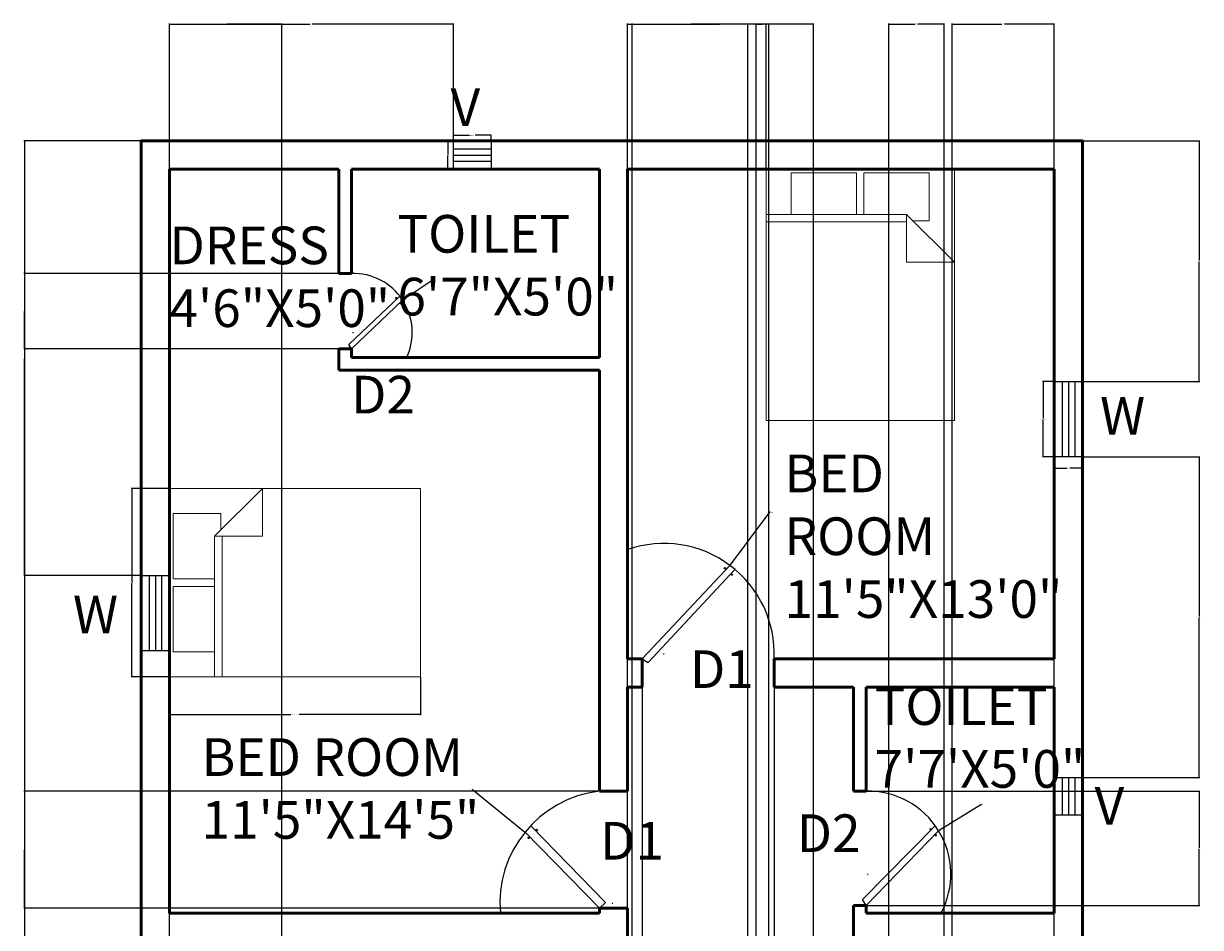
# Model space of a CAD drawing. Units: inches. Extents: x -15 to 361, y -684 to 58.
# Tile 3 of 3: x -15 to 361, y -230 to 58. Entities that reach past the tile are written whole.
import ezdxf

# ---------------------------------------------------------------- set-up
doc = ezdxf.new("R2010")
doc.units = ezdxf.units.IN
doc.header["$MEASUREMENT"] = 0
for name, color, linetype, lineweight in [('A-ANNO-DIMS', 2, 'Continuous', 18), ('A-ANNO-TEXT', 7, 'Continuous', 18), ('A-AREA-IDEN', 7, 'Continuous', 25), ('A-DOOR', 3, 'Continuous', 25), ('A-FURN', 8, 'Continuous', 18), ('A-GLAZ', 4, 'Continuous', 25), ('A-WALL', 7, 'Continuous', 50)]:
    doc.layers.add(name, color=color, linetype=linetype, lineweight=lineweight)
doc.styles.get("Standard").update_dxf_attribs({"font": 'arial.ttf'})
doc.dimstyles.get("Standard").update_dxf_attribs({"dimtxt": 0.18, "dimasz": 0.18, "dimexe": 0.18, "dimexo": 0.0625, "dimgap": 0.09, "dimtad": 0, "dimtih": 1, "dimtoh": 1, "dimdec": 4, "dimzin": 0, "dimdsep": 46, "dimtxsty": 'Standard', "dimcen": 0.09, "dimadec": 0, "dimazin": 0, "dimtfac": 1, "dimtdec": 4, "dimtofl": 0, "dimtmove": 0, "dimatfit": 3, "dimfxl": 1, "dimtolj": 1, "dimtzin": 0, "dimarcsym": 0})

# ---------------------------------------------------------------- blocks, each defined once
blk = doc.blocks.new('Bed - Queen')
for p, q in [((0, -80.00003), (0, 0)), ((0, 0), (59.99999, 0)), ((59.99999, 0), (59.99999, -80.00003)), ((7.99999, -1.2), (28.79998, -1.2)), ((7.99999, -14.4), (7.99999, -1.2)), ((28.79998, -1.2), (28.79998, -14.4)), ((31.19999, -1.2), (51.99999, -1.2)), ((31.19999, -14.4), (31.19999, -1.2)), ((51.99999, -1.2), (51.99999, -16.4)), ((0, -14.4), (44.8, -14.4)), ((59.99999, -29.6), (44.8, -14.4)), ((44.8, -14.4), (44.8, -29.6)), ((44.8, -16.8), (0, -16.8)), ((51.99999, -16.4), (46.79936, -16.4)), ((44.8, -29.6), (59.99999, -29.6)), ((59.99999, -80.00003), (0, -80.00003))]:
    blk.add_line(p, q)
blk = doc.blocks.new('WIN-24IN')
for p, q in [((0, 6.5), (24, 6.5)), ((0, 4.5), (24, 4.5)), ((0, 2.5), (24, 2.5))]:
    blk.add_line(p, q)
blk.add_lwpolyline([(0, 9), (24, 9), (24, 0), (0, 0)], close=True)
blk = doc.blocks.new('VENT-12IN')
for p, q in [((0, 6.5), (12, 6.5)), ((0, 4.5), (12, 4.5)), ((0, 2.5), (12, 2.5))]:
    blk.add_line(p, q)
blk.add_lwpolyline([(0, 9), (12, 9), (12, 0), (0, 0)], close=True)
blk = doc.blocks.new('*D9')
at = {"layer": 'A-ANNO-DIMS', "color": 0, "lineweight": -2, "transparency": 16777216}
for p, q in [((313.87, -56.3), (310.15, -56.3)), ((310.33, -56.48), (310.33, -68.12)), ((310.33, -80.12), (310.33, -68.48)), ((313.87, -80.3), (310.15, -80.3))]:
    blk.add_line(p, q, dxfattribs=at)
at = {"layer": 'A-ANNO-DIMS', "color": 0, "transparency": 16777216}
for points in [[(310.3, -56.48), (310.36, -56.48), (310.33, -56.3)], [(310.3, -80.12), (310.36, -80.12), (310.33, -80.3)]]:
    blk.add_solid(points, dxfattribs=at)
at = {"layer": 'Defpoints', "color": 0, "transparency": 16777216}
for p in [(313.93, -56.3), (310.33, -80.3), (313.93, -80.3)]:
    blk.add_point(p, dxfattribs=at)
at = {"layer": 'A-ANNO-DIMS', "color": 0, "transparency": 16777216, "insert": (310.33, -68.3), "char_height": 0.18, "attachment_point": 5}
blk.add_mtext('\\A1;WINDOW 24 TYP.', dxfattribs=at)
blk = doc.blocks.new('*D10')
at = {"layer": 'A-ANNO-DIMS', "color": 0, "lineweight": -2, "transparency": 16777216}
for p, q in [((313.93, -80.36), (313.93, -84.08)), ((322.93, -80.36), (322.93, -84.08)), ((314.11, -83.9), (317.97, -83.9)), ((322.75, -83.9), (318.89, -83.9))]:
    blk.add_line(p, q, dxfattribs=at)
at = {"layer": 'A-ANNO-DIMS', "color": 0, "transparency": 16777216}
for points in [[(314.11, -83.87), (314.11, -83.93), (313.93, -83.9)], [(322.75, -83.87), (322.75, -83.93), (322.93, -83.9)]]:
    blk.add_solid(points, dxfattribs=at)
at = {"layer": 'Defpoints', "color": 0, "transparency": 16777216}
for p in [(313.93, -80.3), (322.93, -80.3), (322.93, -83.9)]:
    blk.add_point(p, dxfattribs=at)
at = {"layer": 'A-ANNO-DIMS', "color": 0, "transparency": 16777216, "insert": (318.43, -83.9), "char_height": 0.18, "attachment_point": 5}
blk.add_mtext('\\A1;9 TYP.', dxfattribs=at)
blk = doc.blocks.new('*D11')
at = {"layer": 'A-ANNO-DIMS', "color": 0, "lineweight": -2, "transparency": 16777216}
for p, q in [((122.4, 20.37), (122.4, 22.29)), ((122.58, 22.11), (127.5, 22.11)), ((134.22, 22.11), (129.31, 22.11)), ((134.4, 20.37), (134.4, 22.29))]:
    blk.add_line(p, q, dxfattribs=at)
at = {"layer": 'A-ANNO-DIMS', "color": 0, "transparency": 16777216}
for points in [[(122.58, 22.14), (122.58, 22.08), (122.4, 22.11)], [(134.22, 22.14), (134.22, 22.08), (134.4, 22.11)]]:
    blk.add_solid(points, dxfattribs=at)
at = {"layer": 'Defpoints', "color": 0, "transparency": 16777216}
for p in [(122.4, 20.31), (134.4, 22.11), (134.4, 20.31)]:
    blk.add_point(p, dxfattribs=at)
at = {"layer": 'A-ANNO-DIMS', "color": 0, "transparency": 16777216, "insert": (128.4, 22.11), "char_height": 0.18, "attachment_point": 5}
blk.add_mtext('\\A1;VENT 12 TYP.', dxfattribs=at)
blk = doc.blocks.new('*D12')
at = {"layer": 'A-ANNO-DIMS', "color": 0, "lineweight": -2, "transparency": 16777216}
for p, q in [((122.34, 20.31), (120.42, 20.31)), ((120.6, 20.13), (120.6, 15.99)), ((120.6, 11.49), (120.6, 15.63)), ((122.34, 11.31), (120.42, 11.31))]:
    blk.add_line(p, q, dxfattribs=at)
at = {"layer": 'A-ANNO-DIMS', "color": 0, "transparency": 16777216}
for points in [[(120.57, 20.13), (120.63, 20.13), (120.6, 20.31)], [(120.57, 11.49), (120.63, 11.49), (120.6, 11.31)]]:
    blk.add_solid(points, dxfattribs=at)
at = {"layer": 'Defpoints', "color": 0, "transparency": 16777216}
for p in [(120.6, 20.31), (122.4, 20.31), (122.4, 11.31)]:
    blk.add_point(p, dxfattribs=at)
at = {"layer": 'A-ANNO-DIMS', "color": 0, "transparency": 16777216, "insert": (120.6, 15.81), "char_height": 0.18, "attachment_point": 5}
blk.add_mtext('\\A1;9 TYP.', dxfattribs=at)
blk = doc.blocks.new('*D13')
at = {"layer": 'A-ANNO-DIMS', "color": 0, "lineweight": -2, "transparency": 16777216}
for p, q in [((31.93, -150.43), (31.93, -162.55)), ((111.93, -150.43), (111.93, -162.55)), ((32.11, -162.37), (70.62, -162.37)), ((111.75, -162.37), (73.23, -162.37))]:
    blk.add_line(p, q, dxfattribs=at)
at = {"layer": 'A-ANNO-DIMS', "color": 0, "transparency": 16777216}
for points in [[(32.11, -162.34), (32.11, -162.4), (31.93, -162.37)], [(111.75, -162.34), (111.75, -162.4), (111.93, -162.37)]]:
    blk.add_solid(points, dxfattribs=at)
at = {"layer": 'Defpoints', "color": 0, "transparency": 16777216}
for p in [(31.93, -150.37), (111.93, -150.37), (31.93, -162.37)]:
    blk.add_point(p, dxfattribs=at)
at = {"layer": 'A-ANNO-DIMS', "color": 0, "transparency": 16777216, "insert": (71.93, -162.37), "char_height": 0.18, "attachment_point": 5}
blk.add_mtext('\\A1;QUEEN BED 80 TYP.', dxfattribs=at)
blk = doc.blocks.new('*D14')
at = {"layer": 'A-ANNO-DIMS', "color": 0, "lineweight": -2, "transparency": 16777216}
for p, q in [((31.87, -90.37), (19.75, -90.37)), ((19.93, -90.55), (19.93, -120.18)), ((19.93, -150.19), (19.93, -120.55)), ((31.87, -150.37), (19.75, -150.37))]:
    blk.add_line(p, q, dxfattribs=at)
at = {"layer": 'A-ANNO-DIMS', "color": 0, "transparency": 16777216}
for points in [[(19.9, -90.55), (19.96, -90.55), (19.93, -90.37)], [(19.9, -150.19), (19.96, -150.19), (19.93, -150.37)]]:
    blk.add_solid(points, dxfattribs=at)
at = {"layer": 'Defpoints', "color": 0, "transparency": 16777216}
for p in [(19.93, -90.37), (31.93, -90.37), (31.93, -150.37)]:
    blk.add_point(p, dxfattribs=at)
at = {"layer": 'A-ANNO-DIMS', "color": 0, "transparency": 16777216, "insert": (19.93, -120.37), "char_height": 0.18, "attachment_point": 5}
blk.add_mtext('\\A1;60 TYP.', dxfattribs=at)
blk = doc.blocks.new('*D24')
at = {"layer": 'A-ANNO-DIMS', "color": 0, "lineweight": -2, "transparency": 16777216}
for p, q in [((22.87, 20.31), (-14.45, 20.31)), ((-14.27, 20.13), (-14.27, -309.51)), ((-14.27, -639.51), (-14.27, -309.87)), ((22.87, -639.69), (-14.45, -639.69))]:
    blk.add_line(p, q, dxfattribs=at)
at = {"layer": 'A-ANNO-DIMS', "color": 0, "transparency": 16777216}
for points in [[(-14.3, 20.13), (-14.24, 20.13), (-14.27, 20.31)], [(-14.3, -639.51), (-14.24, -639.51), (-14.27, -639.69)]]:
    blk.add_solid(points, dxfattribs=at)
at = {"layer": 'Defpoints', "color": 0, "transparency": 16777216}
for p in [(-14.27, 20.31), (22.93, 20.31), (22.93, -639.69)]:
    blk.add_point(p, dxfattribs=at)
at = {"layer": 'A-ANNO-DIMS', "color": 0, "transparency": 16777216, "insert": (-14.27, -309.69), "char_height": 0.18, "attachment_point": 5}
blk.add_mtext('\\A1;660', dxfattribs=at)
blk = doc.blocks.new('*D25')
at = {"layer": 'A-ANNO-DIMS', "color": 0, "lineweight": -2, "transparency": 16777216}
for p, q in [((31.93, 11.37), (31.93, 57.69)), ((32.11, 57.51), (76.77, 57.51)), ((122.22, 57.51), (77.56, 57.51)), ((122.4, 11.37), (122.4, 57.69))]:
    blk.add_line(p, q, dxfattribs=at)
at = {"layer": 'A-ANNO-DIMS', "color": 0, "transparency": 16777216}
for points in [[(32.11, 57.54), (32.11, 57.48), (31.93, 57.51)], [(122.22, 57.54), (122.22, 57.48), (122.4, 57.51)]]:
    blk.add_solid(points, dxfattribs=at)
at = {"layer": 'Defpoints', "color": 0, "transparency": 16777216}
for p in [(122.4, 57.51), (31.93, 11.31), (122.4, 11.31)]:
    blk.add_point(p, dxfattribs=at)
at = {"layer": 'A-ANNO-DIMS', "color": 0, "transparency": 16777216, "insert": (77.16, 57.51), "char_height": 0.18, "attachment_point": 5}
blk.add_mtext('\\A1;90.47', dxfattribs=at)
blk = doc.blocks.new('*D26')
at = {"layer": 'A-ANNO-DIMS', "color": 0, "lineweight": -2, "transparency": 16777216}
for p, q in [((322.99, 20.31), (360.31, 20.31)), ((360.13, 20.13), (360.13, -17.81)), ((360.13, -56.12), (360.13, -18.18)), ((322.99, -56.3), (360.31, -56.3))]:
    blk.add_line(p, q, dxfattribs=at)
at = {"layer": 'A-ANNO-DIMS', "color": 0, "transparency": 16777216}
for points in [[(360.1, 20.13), (360.16, 20.13), (360.13, 20.31)], [(360.1, -56.12), (360.16, -56.12), (360.13, -56.3)]]:
    blk.add_solid(points, dxfattribs=at)
at = {"layer": 'Defpoints', "color": 0, "transparency": 16777216}
for p in [(322.93, 20.31), (322.93, -56.3), (360.13, -56.3)]:
    blk.add_point(p, dxfattribs=at)
at = {"layer": 'A-ANNO-DIMS', "color": 0, "transparency": 16777216, "insert": (360.13, -18), "char_height": 0.18, "attachment_point": 5}
blk.add_mtext('\\A1;76.61', dxfattribs=at)
blk = doc.blocks.new('*D27')
at = {"layer": 'A-ANNO-DIMS', "color": 0, "lineweight": -2, "transparency": 16777216}
for p, q in [((322.99, -80.3), (360.31, -80.3)), ((360.13, -80.48), (360.13, -131.21)), ((360.13, -182.3), (360.13, -131.57)), ((322.99, -182.48), (360.31, -182.48))]:
    blk.add_line(p, q, dxfattribs=at)
at = {"layer": 'A-ANNO-DIMS', "color": 0, "transparency": 16777216}
for points in [[(360.1, -80.48), (360.16, -80.48), (360.13, -80.3)], [(360.1, -182.3), (360.16, -182.3), (360.13, -182.48)]]:
    blk.add_solid(points, dxfattribs=at)
at = {"layer": 'Defpoints', "color": 0, "transparency": 16777216}
for p in [(322.93, -80.3), (322.93, -182.48), (360.13, -182.48)]:
    blk.add_point(p, dxfattribs=at)
at = {"layer": 'A-ANNO-DIMS', "color": 0, "transparency": 16777216, "insert": (360.13, -131.39), "char_height": 0.18, "attachment_point": 5}
blk.add_mtext('\\A1;102.18', dxfattribs=at)
blk = doc.blocks.new('*D31')
at = {"layer": 'A-ANNO-DIMS', "color": 0, "lineweight": -2, "transparency": 16777216}
for p, q in [((177.93, -549.63), (177.93, 57.69)), ((178.11, 57.51), (207.18, 57.51)), ((237.04, 57.51), (207.97, 57.51)), ((237.22, -549.63), (237.22, 57.69))]:
    blk.add_line(p, q, dxfattribs=at)
at = {"layer": 'A-ANNO-DIMS', "color": 0, "transparency": 16777216}
for points in [[(178.11, 57.54), (178.11, 57.48), (177.93, 57.51)], [(237.04, 57.54), (237.04, 57.48), (237.22, 57.51)]]:
    blk.add_solid(points, dxfattribs=at)
at = {"layer": 'Defpoints', "color": 0, "transparency": 16777216}
for p in [(237.22, 57.51), (177.93, -549.69), (237.22, -549.69)]:
    blk.add_point(p, dxfattribs=at)
at = {"layer": 'A-ANNO-DIMS', "color": 0, "transparency": 16777216, "insert": (207.57, 57.51), "char_height": 0.18, "attachment_point": 5}
blk.add_mtext('\\A1;59.29', dxfattribs=at)
blk = doc.blocks.new('*D32')
at = {"layer": 'A-ANNO-DIMS', "color": 0, "lineweight": -2, "transparency": 16777216}
for p, q in [((31.93, -396.63), (31.93, 57.69)), ((32.11, 57.51), (49.42, 57.51)), ((67.52, 57.51), (50.21, 57.51)), ((67.7, -396.63), (67.7, 57.69))]:
    blk.add_line(p, q, dxfattribs=at)
at = {"layer": 'A-ANNO-DIMS', "color": 0, "transparency": 16777216}
for points in [[(32.11, 57.54), (32.11, 57.48), (31.93, 57.51)], [(67.52, 57.54), (67.52, 57.48), (67.7, 57.51)]]:
    blk.add_solid(points, dxfattribs=at)
at = {"layer": 'Defpoints', "color": 0, "transparency": 16777216}
for p in [(67.7, 57.51), (31.93, -396.69), (67.7, -396.69)]:
    blk.add_point(p, dxfattribs=at)
at = {"layer": 'A-ANNO-DIMS', "color": 0, "transparency": 16777216, "insert": (49.81, 57.51), "char_height": 0.18, "attachment_point": 5}
blk.add_mtext('\\A1;35.77', dxfattribs=at)
blk = doc.blocks.new('*D33')
at = {"layer": 'A-ANNO-DIMS', "color": 0, "lineweight": -2, "transparency": 16777216}
for p, q in [((22.87, 20.31), (-14.45, 20.31)), ((-14.27, 20.13), (-14.27, -48.7)), ((-14.27, -117.9), (-14.27, -49.07)), ((22.87, -118.08), (-14.45, -118.08))]:
    blk.add_line(p, q, dxfattribs=at)
at = {"layer": 'A-ANNO-DIMS', "color": 0, "transparency": 16777216}
for points in [[(-14.3, 20.13), (-14.24, 20.13), (-14.27, 20.31)], [(-14.3, -117.9), (-14.24, -117.9), (-14.27, -118.08)]]:
    blk.add_solid(points, dxfattribs=at)
at = {"layer": 'Defpoints', "color": 0, "transparency": 16777216}
for p in [(22.93, 20.31), (-14.27, -118.08), (22.93, -118.08)]:
    blk.add_point(p, dxfattribs=at)
at = {"layer": 'A-ANNO-DIMS', "color": 0, "transparency": 16777216, "insert": (-14.27, -48.89), "char_height": 0.18, "attachment_point": 5}
blk.add_mtext('\\A1;138.4', dxfattribs=at)
blk = doc.blocks.new('*D36')
at = {"layer": 'A-ANNO-DIMS', "color": 0, "lineweight": -2, "transparency": 16777216}
for p, q in [((85.87, -21.88), (-14.45, -21.88)), ((-14.27, -22.06), (-14.27, -33.7)), ((-14.27, -45.7), (-14.27, -34.06)), ((85.87, -45.88), (-14.45, -45.88))]:
    blk.add_line(p, q, dxfattribs=at)
at = {"layer": 'A-ANNO-DIMS', "color": 0, "transparency": 16777216}
for points in [[(-14.3, -22.06), (-14.24, -22.06), (-14.27, -21.88)], [(-14.3, -45.7), (-14.24, -45.7), (-14.27, -45.88)]]:
    blk.add_solid(points, dxfattribs=at)
at = {"layer": 'Defpoints', "color": 0, "transparency": 16777216}
for p in [(85.93, -21.88), (-14.27, -45.88), (85.93, -45.88)]:
    blk.add_point(p, dxfattribs=at)
at = {"layer": 'A-ANNO-DIMS', "color": 0, "transparency": 16777216, "insert": (-14.27, -33.88), "char_height": 0.18, "attachment_point": 5}
blk.add_mtext('\\A1;24', dxfattribs=at)
blk = doc.blocks.new('*D37')
at = {"layer": 'A-ANNO-DIMS', "color": 0, "lineweight": -2, "transparency": 16777216}
for p, q in [((182.53, -153.75), (182.53, -677.07)), ((224.64, -153.75), (224.64, -677.07)), ((182.71, -676.89), (203.21, -676.89)), ((224.46, -676.89), (203.97, -676.89))]:
    blk.add_line(p, q, dxfattribs=at)
at = {"layer": 'A-ANNO-DIMS', "color": 0, "transparency": 16777216}
for points in [[(182.71, -676.86), (182.71, -676.92), (182.53, -676.89)], [(224.46, -676.86), (224.46, -676.92), (224.64, -676.89)]]:
    blk.add_solid(points, dxfattribs=at)
at = {"layer": 'Defpoints', "color": 0, "transparency": 16777216}
for p in [(182.53, -153.69), (224.64, -153.69), (224.64, -676.89)]:
    blk.add_point(p, dxfattribs=at)
at = {"layer": 'A-ANNO-DIMS', "color": 0, "transparency": 16777216, "insert": (203.59, -676.89), "char_height": 0.18, "attachment_point": 5}
blk.add_mtext('\\A1;42.11', dxfattribs=at)
blk = doc.blocks.new('*D38')
at = {"layer": 'A-ANNO-DIMS', "color": 0, "lineweight": -2, "transparency": 16777216}
for p, q in [((168.87, -186.78), (-14.45, -186.78)), ((-14.27, -186.96), (-14.27, -205.25)), ((-14.27, -223.91), (-14.27, -205.62)), ((168.87, -224.09), (-14.45, -224.09))]:
    blk.add_line(p, q, dxfattribs=at)
at = {"layer": 'A-ANNO-DIMS', "color": 0, "transparency": 16777216}
for points in [[(-14.3, -186.96), (-14.24, -186.96), (-14.27, -186.78)], [(-14.3, -223.91), (-14.24, -223.91), (-14.27, -224.09)]]:
    blk.add_solid(points, dxfattribs=at)
at = {"layer": 'Defpoints', "color": 0, "transparency": 16777216}
for p in [(168.93, -186.78), (-14.27, -224.09), (168.93, -224.09)]:
    blk.add_point(p, dxfattribs=at)
at = {"layer": 'A-ANNO-DIMS', "color": 0, "transparency": 16777216, "insert": (-14.27, -205.44), "char_height": 0.18, "attachment_point": 5}
blk.add_mtext('\\A1;37.31', dxfattribs=at)
blk = doc.blocks.new('*D39')
at = {"layer": 'A-ANNO-DIMS', "color": 0, "lineweight": -2, "transparency": 16777216}
for p, q in [((253.99, -186.78), (360.31, -186.78)), ((360.13, -186.96), (360.13, -204.81)), ((360.13, -223.02), (360.13, -205.17)), ((253.99, -223.2), (360.31, -223.2))]:
    blk.add_line(p, q, dxfattribs=at)
at = {"layer": 'A-ANNO-DIMS', "color": 0, "transparency": 16777216}
for points in [[(360.1, -186.96), (360.16, -186.96), (360.13, -186.78)], [(360.1, -223.02), (360.16, -223.02), (360.13, -223.2)]]:
    blk.add_solid(points, dxfattribs=at)
at = {"layer": 'Defpoints', "color": 0, "transparency": 16777216}
for p in [(253.93, -186.78), (253.93, -223.2), (360.13, -223.2)]:
    blk.add_point(p, dxfattribs=at)
at = {"layer": 'A-ANNO-DIMS', "color": 0, "transparency": 16777216, "insert": (360.13, -204.99), "char_height": 0.18, "attachment_point": 5}
blk.add_mtext('\\A1;36.42', dxfattribs=at)
blk = doc.blocks.new('*D42')
at = {"layer": 'A-ANNO-DIMS', "color": 0, "lineweight": -2, "transparency": 16777216}
for p, q in [((179.42, -396.63), (179.42, 57.69)), ((179.6, 57.51), (197.42, 57.51)), ((216.02, 57.51), (198.21, 57.51)), ((216.2, -396.63), (216.2, 57.69))]:
    blk.add_line(p, q, dxfattribs=at)
at = {"layer": 'A-ANNO-DIMS', "color": 0, "transparency": 16777216}
for points in [[(179.6, 57.54), (179.6, 57.48), (179.42, 57.51)], [(216.02, 57.54), (216.02, 57.48), (216.2, 57.51)]]:
    blk.add_solid(points, dxfattribs=at)
at = {"layer": 'Defpoints', "color": 0, "transparency": 16777216}
for p in [(216.2, 57.51), (179.42, -396.69), (216.2, -396.69)]:
    blk.add_point(p, dxfattribs=at)
at = {"layer": 'A-ANNO-DIMS', "color": 0, "transparency": 16777216, "insert": (197.81, 57.51), "char_height": 0.18, "attachment_point": 5}
blk.add_mtext('\\A1;36.78', dxfattribs=at)
blk = doc.blocks.new('*D44')
at = {"layer": 'A-ANNO-DIMS', "color": 0, "lineweight": -2, "transparency": 16777216}
for p, q in [((281.35, -558.63), (281.35, 57.69)), ((281.53, 57.51), (297.18, 57.51)), ((313.75, 57.51), (298.1, 57.51)), ((313.93, -558.63), (313.93, 57.69))]:
    blk.add_line(p, q, dxfattribs=at)
at = {"layer": 'A-ANNO-DIMS', "color": 0, "transparency": 16777216}
for points in [[(281.53, 57.54), (281.53, 57.48), (281.35, 57.51)], [(313.75, 57.54), (313.75, 57.48), (313.93, 57.51)]]:
    blk.add_solid(points, dxfattribs=at)
at = {"layer": 'Defpoints', "color": 0, "transparency": 16777216}
for p in [(313.93, 57.51), (281.35, -558.69), (313.93, -558.69)]:
    blk.add_point(p, dxfattribs=at)
at = {"layer": 'A-ANNO-DIMS', "color": 0, "transparency": 16777216, "insert": (297.64, 57.51), "char_height": 0.18, "attachment_point": 5}
blk.add_mtext('\\A1;32.575', dxfattribs=at)
blk = doc.blocks.new('*D49')
at = {"layer": 'A-ANNO-DIMS', "color": 0, "lineweight": -2, "transparency": 16777216}
for p, q in [((218.93, -315.63), (218.93, 57.69)), ((219.11, 57.51), (220.78, 57.51)), ((222.75, 57.51), (221.08, 57.51)), ((222.93, -315.63), (222.93, 57.69))]:
    blk.add_line(p, q, dxfattribs=at)
at = {"layer": 'A-ANNO-DIMS', "color": 0, "transparency": 16777216}
for points in [[(219.11, 57.54), (219.11, 57.48), (218.93, 57.51)], [(222.75, 57.54), (222.75, 57.48), (222.93, 57.51)]]:
    blk.add_solid(points, dxfattribs=at)
at = {"layer": 'Defpoints', "color": 0, "transparency": 16777216}
for p in [(222.93, 57.51), (218.93, -315.69), (222.93, -315.69)]:
    blk.add_point(p, dxfattribs=at)
at = {"layer": 'A-ANNO-DIMS', "color": 0, "transparency": 16777216, "insert": (220.93, 57.51), "char_height": 0.18, "attachment_point": 5}
blk.add_mtext('\\A1;4', dxfattribs=at)
blk = doc.blocks.new('*D51')
at = {"layer": 'A-ANNO-DIMS', "color": 0, "lineweight": -2, "transparency": 16777216}
for p, q in [((177.93, 11.37), (177.93, 57.69)), ((178.11, 57.51), (199.53, 57.51)), ((221.88, 57.51), (200.46, 57.51)), ((222.06, 11.37), (222.06, 57.69))]:
    blk.add_line(p, q, dxfattribs=at)
at = {"layer": 'A-ANNO-DIMS', "color": 0, "transparency": 16777216}
for points in [[(178.11, 57.54), (178.11, 57.48), (177.93, 57.51)], [(221.88, 57.54), (221.88, 57.48), (222.06, 57.51)]]:
    blk.add_solid(points, dxfattribs=at)
at = {"layer": 'Defpoints', "color": 0, "transparency": 16777216}
for p in [(177.93, 57.51), (177.93, 11.31), (222.06, 11.31)]:
    blk.add_point(p, dxfattribs=at)
at = {"layer": 'A-ANNO-DIMS', "color": 0, "transparency": 16777216, "insert": (200, 57.51), "char_height": 0.18, "attachment_point": 5}
blk.add_mtext('\\A1;44.135', dxfattribs=at)
blk = doc.blocks.new('*D52')
at = {"layer": 'A-ANNO-DIMS', "color": 0, "lineweight": -2, "transparency": 16777216}
for p, q in [((261.22, -549.63), (261.22, 57.69)), ((261.4, 57.51), (269.54, 57.51)), ((278.6, 57.51), (270.45, 57.51)), ((278.78, -549.63), (278.78, 57.69))]:
    blk.add_line(p, q, dxfattribs=at)
at = {"layer": 'A-ANNO-DIMS', "color": 0, "transparency": 16777216}
for points in [[(261.4, 57.54), (261.4, 57.48), (261.22, 57.51)], [(278.6, 57.54), (278.6, 57.48), (278.78, 57.51)]]:
    blk.add_solid(points, dxfattribs=at)
at = {"layer": 'Defpoints', "color": 0, "transparency": 16777216}
for p in [(278.78, 57.51), (261.22, -549.69), (278.78, -549.69)]:
    blk.add_point(p, dxfattribs=at)
at = {"layer": 'A-ANNO-DIMS', "color": 0, "transparency": 16777216, "insert": (270, 57.51), "char_height": 0.18, "attachment_point": 5}
blk.add_mtext('\\A1;17.564', dxfattribs=at)
blk = doc.blocks.new('*D53')
at = {"layer": 'A-ANNO-DIMS', "color": 0, "lineweight": -2, "transparency": 16777216}
for p, q in [((115.66, -24.17), (106.36, -30.28)), ((115.84, -24.17), (115.66, -24.17)), ((90.37, -40.72), (90.55, -40.72)), ((90.46, -40.81), (90.46, -40.63))]:
    blk.add_line(p, q, dxfattribs=at)
at = {"layer": 'A-ANNO-DIMS', "color": 0, "transparency": 16777216}
blk.add_solid([(106.35, -30.25), (106.38, -30.3), (106.21, -30.38)], dxfattribs=at)
at = {"layer": 'Defpoints', "color": 0, "transparency": 16777216}
for p in [(106.21, -30.38), (90.46, -40.72)]:
    blk.add_point(p, dxfattribs=at)
at = {"layer": 'A-ANNO-DIMS', "color": 0, "transparency": 16777216, "insert": (116.32, -24.17), "char_height": 0.18, "attachment_point": 5}
blk.add_mtext('\\A1;R18.85', dxfattribs=at)
blk = doc.blocks.new('*D54')
at = {"layer": 'A-ANNO-DIMS', "color": 0, "lineweight": -2, "transparency": 16777216}
for p, q in [((223.15, -97.95), (210.64, -114.73)), ((223.33, -97.95), (223.15, -97.95)), ((189.41, -143.07), (189.59, -143.07)), ((189.5, -143.16), (189.5, -142.98))]:
    blk.add_line(p, q, dxfattribs=at)
at = {"layer": 'A-ANNO-DIMS', "color": 0, "transparency": 16777216}
blk.add_solid([(210.62, -114.71), (210.66, -114.75), (210.53, -114.87)], dxfattribs=at)
at = {"layer": 'Defpoints', "color": 0, "transparency": 16777216}
for p in [(210.53, -114.87), (189.5, -143.07)]:
    blk.add_point(p, dxfattribs=at)
at = {"layer": 'A-ANNO-DIMS', "color": 0, "transparency": 16777216, "insert": (223.88, -97.95), "char_height": 0.18, "attachment_point": 5}
blk.add_mtext('\\A1;R35.174', dxfattribs=at)
blk = doc.blocks.new('*D55')
at = {"layer": 'A-ANNO-DIMS', "color": 0, "lineweight": -2, "transparency": 16777216}
for p, q in [((128.35, -186.27), (128.53, -186.27)), ((128.53, -186.27), (145.11, -199.71)), ((173.03, -222.41), (173.21, -222.41)), ((173.12, -222.5), (173.12, -222.32))]:
    blk.add_line(p, q, dxfattribs=at)
at = {"layer": 'A-ANNO-DIMS', "color": 0, "transparency": 16777216}
blk.add_solid([(145.13, -199.69), (145.09, -199.73), (145.25, -199.82)], dxfattribs=at)
at = {"layer": 'Defpoints', "color": 0, "transparency": 16777216}
for p in [(145.25, -199.82), (173.12, -222.41)]:
    blk.add_point(p, dxfattribs=at)
at = {"layer": 'A-ANNO-DIMS', "color": 0, "transparency": 16777216, "insert": (127.87, -186.27), "char_height": 0.18, "attachment_point": 5}
blk.add_mtext('\\A1;R35.87', dxfattribs=at)
blk = doc.blocks.new('*D56')
at = {"layer": 'A-ANNO-DIMS', "color": 0, "lineweight": -2, "transparency": 16777216}
for p, q in [((290.56, -191.09), (277.2, -199.28)), ((290.74, -191.09), (290.56, -191.09)), ((254.45, -213.19), (254.63, -213.19)), ((254.54, -213.28), (254.54, -213.1))]:
    blk.add_line(p, q, dxfattribs=at)
at = {"layer": 'A-ANNO-DIMS', "color": 0, "transparency": 16777216}
blk.add_solid([(277.19, -199.25), (277.22, -199.31), (277.05, -199.37)], dxfattribs=at)
at = {"layer": 'Defpoints', "color": 0, "transparency": 16777216}
for p in [(277.05, -199.37), (254.54, -213.19)]:
    blk.add_point(p, dxfattribs=at)
at = {"layer": 'A-ANNO-DIMS', "color": 0, "transparency": 16777216, "insert": (291.2, -191.09), "char_height": 0.18, "attachment_point": 5}
blk.add_mtext('\\A1;R26.41', dxfattribs=at)

msp = doc.modelspace()

# ---------------------------------------------------------------- linework, layer by layer
at = {"layer": 'A-DOOR'}
for p, q in [((89.1438, -44.5251), (105.3486, -29.168)), ((106.2116, -30.3753), (89.9279, -45.8832)), ((89.9279, -45.8832), (89.1438, -44.5251)), ((210.5325, -114.8732), (182.5334, -144.6922)), ((184.525, -145.8421), (212.1418, -116.1481)), ((182.5334, -144.6922), (184.525, -145.8421)), ((147.1828, -197.9368), (147.0275, -197.7903)), ((170.8619, -222.2048), (147.1828, -197.9368)), ((252.8272, -221.2941), (276.0063, -197.8023)), ((145.2487, -199.8239), (168.9279, -224.0919)), ((277.0497, -199.3742), (253.9279, -223.2006)), ((253.9279, -223.2006), (252.8272, -221.2941)), ((168.9279, -224.0919), (170.8619, -222.2048)), ((168.9279, -224.0919), (168.9279, -224.0919))]:
    msp.add_line(p, q, dxfattribs=at)
for centre in [(104.2383, -29.7367), (105.6816, -31.4891), (208.9468, -115.7782), (211.0586, -117.8299), (274.5016, -198.8892), (146.4034, -201.6798), (148.9639, -199.1583), (276.0914, -200.8162)]:
    msp.add_circle(centre, 0.216, dxfattribs=at)
for centre, radius, start, end in [((90.4581, -40.7247), 18.849, 334.994791, 91.612067), ((189.5048, -143.0699), 35.1742, 357.356475, 109.21602), ((173.1201, -222.4088), 35.8732, 96.711004, 185.25156), ((254.5378, -213.1851), 26.4108, 331.734156, 91.323318)]:
    msp.add_arc(centre, radius, start, end, dxfattribs=at)
at = {"layer": 'A-WALL'}
for p, q in [((31.9279, 11.3078), (85.9279, 11.3078)), ((31.9279, -225.6922), (31.9279, 11.3078)), ((85.9279, -21.8832), (85.9279, 11.3078)), ((89.9279, -21.8832), (89.9279, 11.3078)), ((89.9279, 11.3078), (168.9279, 11.3078)), ((168.9279, -48.6922), (168.9279, 11.3078)), ((177.9279, -144.6922), (177.9279, 11.3078)), ((177.9279, 11.3078), (313.9279, 11.3078)), ((313.9279, 11.3078), (313.9279, -144.6922)), ((85.9279, -21.8832), (89.9279, -21.8832)), ((85.9279, -52.6922), (85.9279, -45.8832)), ((85.9279, -45.8832), (89.9279, -45.8832)), ((89.9279, -48.6922), (89.9279, -45.8832)), ((89.9279, -48.6922), (168.9279, -48.6922)), ((85.9279, -52.6922), (168.9279, -52.6922)), ((168.9279, -186.7813), (168.9279, -52.6922)), ((177.9279, -144.6922), (182.5334, -144.6922)), ((182.5334, -144.6922), (182.5334, -153.6922)), ((249.9279, -144.6922), (224.6415, -144.6922)), ((224.6415, -144.6922), (224.6415, -153.6922)), ((249.9279, -144.6922), (313.9279, -144.6922)), ((177.9279, -186.7813), (177.9279, -153.6922)), ((182.5334, -153.6922), (177.9279, -153.6922)), ((224.6415, -153.6922), (249.9279, -153.6922)), ((249.9279, -153.6922), (249.9279, -186.7813)), ((253.9279, -153.6922), (253.9279, -186.7813)), ((253.9279, -153.6922), (313.9279, -153.6922)), ((313.9279, -153.6922), (313.9279, -225.6922)), ((168.9279, -186.7813), (177.9279, -186.7813)), ((249.9279, -186.7813), (253.9279, -186.7813)), ((168.9279, -225.6922), (168.9279, -224.0919)), ((168.9279, -224.0919), (177.9279, -224.0919)), ((177.9279, -225.6922), (177.9279, -224.0919)), ((249.9279, -223.2006), (253.9279, -223.2006)), ((249.9279, -223.2006), (249.9279, -234.6922)), ((253.9279, -223.2006), (253.9279, -225.6922)), ((31.9279, -225.6922), (168.9279, -225.6922)), ((177.9279, -225.6922), (177.9279, -234.6922)), ((253.9279, -225.6922), (313.9279, -225.6922))]:
    msp.add_line(p, q, dxfattribs=at)
msp.add_lwpolyline([(31.9279, -639.6922), (22.9279, -639.6922), (22.9279, 20.3078), (322.9279, 20.3078), (322.9279, -639.6922), (137.4946, -639.6922)], dxfattribs=at)

# ---------------------------------------------------------------- block references
at = {"layer": 'A-FURN'}
msp.add_blockref('Bed - Queen', (222.0631, 11.3078), dxfattribs=at)
at = {"layer": 'A-FURN', "rotation": 90}
msp.add_blockref('Bed - Queen', (31.9279, -150.3662), dxfattribs=at)
at = {"layer": 'A-GLAZ'}
msp.add_blockref('VENT-12IN', (122.402, 11.308), dxfattribs=at)
for name, p, rotation in [('WIN-24IN', (313.9281, -56.2999), 270.0000000000002), ('WIN-24IN', (22.9281, -118.0792), 270.0000000000003), ('VENT-12IN', (313.9281, -182.476), 269.9999999999999)]:
    msp.add_blockref(name, p, dxfattribs=dict(at, rotation=rotation))

# ---------------------------------------------------------------- texts
at = {"layer": 'A-ANNO-TEXT', "char_height": 12, "attachment_point": 1}
for s, width, insert in [('V', 16.992712, (121.5185, 37.0177)), ('D2 ', 41.238406, (89.8, -54.5048)), ('W', 26.464345, (328.5039, -61.2404)), ('W', 16.576755, (1.1732, -124.5502)), ('D1', 13.187109, (197.8078, -141.9253)), ('V', 6.866057, (326.7774, -185.4845)), ('D2', 20.185882, (231.813, -194.1876)), ('D1', 18.378187, (169.1464, -196.595))]:
    msp.add_mtext_dynamic_manual_height_columns(s, width=width, gutter_width=60, heights=[0], dxfattribs=dict(at, insert=insert))
at = {"layer": 'A-AREA-IDEN', "char_height": 12, "attachment_point": 1}
for s, width, insert in [('TOILET\\P6\'7"X5\'0"', 64.364168, (104.5637, -3.2803)), ('DRESS\\P4\'6"X5\'0"', 35.025429, (31.9279, -6.9585)), ('BED ROOM\\P11\'5"X13\'0"', 79.916411, (227.9611, -79.5933)), ('TOILET\\P7\'7\'X5\'0"', 42.696992, (256.6652, -153.6922)), ('BED ROOM\\P11\'5"X14\'5"', 97.180912, (42.1661, -169.9362))]:
    msp.add_mtext_dynamic_manual_height_columns(s, width=width, gutter_width=60, heights=[0], dxfattribs=dict(at, insert=insert))

# ---------------------------------------------------------------- dimensions: what is measured, and where the dimension line sits
at = {"layer": 'A-ANNO-DIMS'}
for base, p1, p2, override, picture, middle in [((122.402, 57.5078), (31.9279, 11.3078), (122.402, 11.3078), {"dimdec": 2, "dimlfac": 1, "dimrnd": 0, "dimzin": 0, "dimdsep": 46, "dimlunit": 2}, '*D25', (77.1649, 57.5078)), ((67.6973, 57.5078), (31.9279, -396.6922), (67.6973, -396.6922), {"dimdec": 2, "dimlfac": 1, "dimrnd": 0, "dimzin": 0, "dimdsep": 46, "dimlunit": 2}, '*D32', (49.8126, 57.5078)), ((237.2164, 57.5078), (177.9279, -549.6922), (237.2164, -549.6922), {"dimdec": 2, "dimlfac": 1, "dimrnd": 0, "dimzin": 0, "dimdsep": 46, "dimlunit": 2}, '*D31', (207.5721, 57.5078)), ((177.9279, 57.5078), (222.0631, 11.3078), (177.9279, 11.3078), {"dimdec": 3, "dimlfac": 1, "dimrnd": 0, "dimzin": 0, "dimdsep": 46, "dimlunit": 2}, '*D51', (199.9955, 57.5078)), ((216.2043, 57.5078), (179.4234, -396.6922), (216.2043, -396.6922), {"dimdec": 2, "dimlfac": 1, "dimrnd": 0, "dimzin": 0, "dimdsep": 46, "dimlunit": 2}, '*D42', (197.8139, 57.5078)), ((222.9279, 57.5078), (218.9279, -315.6922), (222.9279, -315.6922), {"dimdec": 0, "dimlfac": 1, "dimrnd": 0, "dimzin": 0, "dimdsep": 46, "dimlunit": 2}, '*D49', (220.9279, 57.5078)), ((278.78086, 57.50778), (261.21639, -549.69222), (278.78086, -549.69222), {"dimdec": 3, "dimlfac": 1, "dimrnd": 0, "dimzin": 0, "dimdsep": 46, "dimlunit": 2}, '*D52', (269.99863, 57.50778)), ((313.9279, 57.5078), (281.3528, -558.6922), (313.9279, -558.6922), {"dimdec": 3, "dimlfac": 1, "dimrnd": 0, "dimzin": 0, "dimdsep": 46, "dimlunit": 2}, '*D44', (297.6403, 57.5078)), ((224.6415, -676.8922), (182.5334, -153.6922), (224.6415, -153.6922), {"dimdec": 2, "dimlfac": 1, "dimrnd": 0, "dimzin": 0, "dimdsep": 46, "dimlunit": 2}, '*D37', (203.5874, -676.8922))]:
    dim = msp.add_linear_dim(base=base, p1=p1, p2=p2, dimstyle='Standard', override=override, dxfattribs=at)
    dim.commit()
    dim.dimension.update_dxf_attribs({"geometry": picture, "text_midpoint": middle})
dim = msp.add_linear_dim(base=(134.402, 22.1078), p1=(122.402, 20.3078), p2=(134.402, 20.3078), text='VENT <> TYP.', dimstyle='Standard', override={"dimdec": 0, "dimlfac": 1, "dimrnd": 0, "dimzin": 0, "dimdsep": 46, "dimlunit": 2}, dxfattribs=at)
dim.commit()
dim.dimension.update_dxf_attribs({"geometry": '*D11', "text_midpoint": (128.402, 22.1078)})
for base, p1, p2, override, picture, middle in [((-14.2721, -118.0796), (22.9279, 20.3078), (22.9279, -118.0796), {"dimdec": 1, "dimlfac": 1, "dimrnd": 0, "dimzin": 0, "dimdsep": 46, "dimlunit": 2}, '*D33', (-14.2721, -48.8859)), ((-14.2721, 20.3078), (22.9279, -639.6922), (22.9279, 20.3078), {"dimdec": 0, "dimlfac": 1, "dimrnd": 0, "dimzin": 0, "dimdsep": 46, "dimlunit": 2}, '*D24', (-14.2721, -309.6922)), ((360.1279, -56.3003), (322.9279, 20.3078), (322.9279, -56.3003), {"dimdec": 2, "dimlfac": 1, "dimrnd": 0, "dimzin": 0, "dimdsep": 46, "dimlunit": 2}, '*D26', (360.1279, -17.9962)), ((-14.2721, -45.8832), (85.9279, -21.8832), (85.9279, -45.8832), {"dimdec": 0, "dimlfac": 1, "dimrnd": 0, "dimzin": 0, "dimdsep": 46, "dimlunit": 2}, '*D36', (-14.2721, -33.8832)), ((360.1279, -182.476), (322.9279, -80.3003), (322.9279, -182.476), {"dimdec": 2, "dimlfac": 1, "dimrnd": 0, "dimzin": 0, "dimdsep": 46, "dimlunit": 2}, '*D27', (360.1279, -131.3882)), ((-14.2721, -224.0919), (168.9279, -186.7813), (168.9279, -224.0919), {"dimdec": 2, "dimlfac": 1, "dimrnd": 0, "dimzin": 0, "dimdsep": 46, "dimlunit": 2}, '*D38', (-14.2721, -205.4366)), ((360.1279, -223.2006), (253.9279, -186.7813), (253.9279, -223.2006), {"dimdec": 2, "dimlfac": 1, "dimrnd": 0, "dimzin": 0, "dimdsep": 46, "dimlunit": 2}, '*D39', (360.1279, -204.991))]:
    dim = msp.add_linear_dim(base=base, p1=p1, p2=p2, angle=90, dimstyle='Standard', override=override, dxfattribs=at)
    dim.commit()
    dim.dimension.update_dxf_attribs({"geometry": picture, "text_midpoint": middle})
for base, p1, p2, angle, text, picture, middle in [((120.602, 20.3078), (122.402, 11.3078), (122.402, 20.3078), 90, '<> TYP.', '*D12', (120.602, 15.8078)), ((310.3279, -80.3003), (313.9279, -56.3003), (313.9279, -80.3003), 270, 'WINDOW <> TYP.', '*D9', (310.3279, -68.3003)), ((322.9279, -83.9003), (313.9279, -80.3003), (322.9279, -80.3003), 0, '<> TYP.', '*D10', (318.4279, -83.9003)), ((19.9279, -90.3662), (31.9279, -150.3662), (31.9279, -90.3662), 90, '<> TYP.', '*D14', (19.9279, -120.3662)), ((31.9279, -162.3662), (111.9279, -150.3662), (31.9279, -150.3662), 180, 'QUEEN BED <> TYP.', '*D13', (71.9279, -162.3662))]:
    dim = msp.add_linear_dim(base=base, p1=p1, p2=p2, angle=angle, text=text, dimstyle='Standard', override={"dimdec": 0, "dimlfac": 1, "dimrnd": 0, "dimzin": 0, "dimdsep": 46, "dimlunit": 2}, dxfattribs=at)
    dim.commit()
    dim.dimension.update_dxf_attribs({"geometry": picture, "text_midpoint": middle})
for center, mpoint, override, picture, middle in [((90.4581, -40.7247), (106.2116, -30.3752), {"dimdec": 2, "dimlfac": 1, "dimrnd": 0, "dimzin": 0, "dimdsep": 46, "dimlunit": 2}, '*D53', (116.3242, -24.1655)), ((189.5048, -143.0699), (210.5321, -114.8729), {"dimdec": 3, "dimlfac": 1, "dimrnd": 0, "dimzin": 0, "dimdsep": 46, "dimlunit": 2}, '*D54', (223.8779, -97.9547)), ((173.1201, -222.4088), (145.2488, -199.8238), {"dimdec": 2, "dimlfac": 1, "dimrnd": 0, "dimzin": 0, "dimdsep": 46, "dimlunit": 2}, '*D55', (127.8662, -186.2728)), ((254.5378, -213.1851), (277.0497, -199.3742), {"dimdec": 2, "dimlfac": 1, "dimrnd": 0, "dimzin": 0, "dimdsep": 46, "dimlunit": 2}, '*D56', (291.1994, -191.0876))]:
    dim = msp.add_radius_dim(center=center, mpoint=mpoint, dimstyle='Standard', override=override, dxfattribs=at)
    dim.commit()
    dim.dimension.update_dxf_attribs({"geometry": picture, "text_midpoint": middle, "dimtype": 164})

doc.saveas('drawing.dxf')
